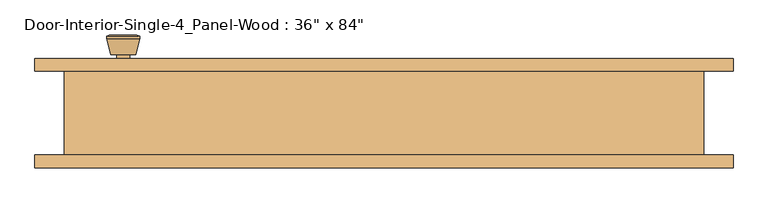
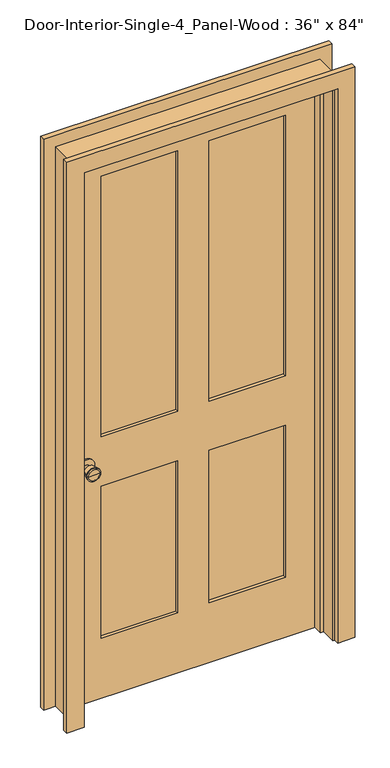
"""IFC4 building model written with IfcOpenShell, lengths in millimetres: door geometry."""

from ifc_helpers import new_model, si_unit, point, frame, frame_2d, origin, place, context, project, spatial, polyline, circle_curve, trimmed, segment, composite_curve, outline, extrude, faceted_brep, source, transform, mapped, element, save
from ifc_brep_helpers import plane_surface, cylinder_surface, revolved_surface, advanced_brep


def door_68a706ac(model_context):
    return source(origin(), model_context, "Body", "SolidModel", [
        advanced_brep(
        [(-393.7, 19.4, 914.4), (-383.7, 19.4, 914.4), (-403.7, 19.4, 914.4), (-373.2241324, -29.6, 914.4), (-393.7, -29.6, 914.4), (-414.1758676, -29.6, 914.4), (-368.7, -27.7721319, 914.4), (-418.7, -27.7721319, 914.4), (-368.7, -24.3084537, 914.4), (-418.7, -24.3084537, 914.4), (-375.063764, 0.4, 914.4), (-412.336236, 0.4, 914.4), (-383.7, 0.4, 914.4), (-403.7, 0.4, 914.4)],
        [
            (0, 1),
            (1, 2, circle_curve(frame((-393.7, 19.4, 914.4), z_axis=(0.0, 1.0, 0.0), x_axis=(-1.0, 0.0, 0.0)), 10.0)),
            (2, 0),
            (2, 1, circle_curve(frame((-393.7, 19.4, 914.4), z_axis=(0.0, 1.0, 0.0), x_axis=(-1.0, 0.0, 0.0)), 10.0)),
            (3, 4),
            (4, 5),
            (5, 3, circle_curve(frame((-393.7, -29.6, 914.4), z_axis=(0.0, -1.0, 0.0), x_axis=(-1.0, 0.0, 0.0)), 20.4758676)),
            (3, 5, circle_curve(frame((-393.7, -29.6, 914.4), z_axis=(0.0, -1.0, 0.0), x_axis=(-1.0, 0.0, 0.0)), 20.4758676)),
            (6, 3),
            (5, 7),
            (7, 6, circle_curve(frame((-393.7, -27.7721319, 914.4), z_axis=(0.0, -1.0, 0.0), x_axis=(-1.0, 0.0, 0.0)), 25.0)),
            (6, 7, circle_curve(frame((-393.7, -27.7721319, 914.4), z_axis=(0.0, -1.0, 0.0), x_axis=(-1.0, 0.0, 0.0)), 25.0)),
            (8, 6),
            (7, 9),
            (9, 8, circle_curve(frame((-393.7, -24.3084537, 914.4), z_axis=(0.0, -1.0, 0.0), x_axis=(-1.0, 0.0, 0.0)), 25.0)),
            (8, 9, circle_curve(frame((-393.7, -24.3084537, 914.4), z_axis=(0.0, -1.0, 0.0), x_axis=(-1.0, 0.0, 0.0)), 25.0)),
            (10, 8),
            (9, 11),
            (11, 10, circle_curve(frame((-393.7, 0.4, 914.4), z_axis=(0.0, -1.0, 0.0), x_axis=(-1.0, 0.0, 0.0)), 18.636236)),
            (10, 11, circle_curve(frame((-393.7, 0.4, 914.4), z_axis=(0.0, -1.0, 0.0), x_axis=(-1.0, 0.0, 0.0)), 18.636236)),
            (12, 10),
            (11, 13),
            (13, 12, circle_curve(frame((-393.7, 0.4, 914.4), z_axis=(0.0, -1.0, 0.0), x_axis=(-1.0, 0.0, 0.0)), 10.0)),
            (12, 13, circle_curve(frame((-393.7, 0.4, 914.4), z_axis=(0.0, -1.0, 0.0), x_axis=(-1.0, 0.0, 0.0)), 10.0)),
            (1, 12),
            (13, 2),
        ],
        [
            plane_surface(frame((-393.7, 19.4, 914.4), z_axis=(0.0, 1.0, 0.0), x_axis=(-1.0, 0.0, 0.0))),
            plane_surface(frame((-393.7, -29.6, 914.4), z_axis=(0.0, -1.0, 0.0), x_axis=(-1.0, 0.0, 0.0))),
            revolved_surface(polyline([(-414.1758676, -29.6, 914.4), (-418.7, -27.7721319, 914.4)]), (-393.7, 19.4, 914.4), (0.0, 1.0, 0.0)),
            cylinder_surface(frame((-393.7, 19.4, 914.4), z_axis=(0.0, 1.0, 0.0), x_axis=(-1.0, 0.0, 0.0)), 25.0),
            revolved_surface(polyline([(-418.7, -24.3084537, 914.4), (-412.336236, 0.4, 914.4)]), (-393.7, 19.4, 914.4), (0.0, 1.0, 0.0)),
            plane_surface(frame((-393.7, 0.4, 914.4), z_axis=(0.0, 1.0, 0.0), x_axis=(-1.0, 0.0, 0.0))),
            cylinder_surface(frame((-393.7, 19.4, 914.4), z_axis=(0.0, 1.0, 0.0), x_axis=(-1.0, 0.0, 0.0)), 10.0),
        ],
        [
            (0, [[1, 2, 3]]),
            (0, [[-3, 4, -1]]),
            (1, [[5, 6, 7]]),
            (1, [[-6, -5, 8]]),
            (2, [[9, -7, 10, 11]]),
            (2, [[-10, -8, -9, 12]]),
            (3, [[13, -11, 14, 15]]),
            (3, [[-14, -12, -13, 16]]),
            (4, [[17, -15, 18, 19]]),
            (4, [[-18, -16, -17, 20]]),
            (5, [[21, -19, 22, 23]]),
            (5, [[-22, -20, -21, 24]]),
            (6, [[25, -23, 26, -2]]),
            (6, [[-26, -24, -25, -4]]),
        ],
    ),
        extrude(outline(composite_curve([segment(trimmed(circle_curve(frame_2d((914.4, -393.7)), 30.0), [point((914.4, -423.7))], [point((914.4, -363.7))], False, "CARTESIAN"), True, "CONTINUOUS"), segment(trimmed(circle_curve(frame_2d((914.4, -393.7)), 30.0), [point((914.4, -363.7))], [point((914.4, -423.7))], False, "CARTESIAN"), True, "CONTINUOUS")], self_intersect=False)), frame((0.0, 19.4, 0.0), z_axis=(0.0, 1.0, 0.0), x_axis=(0.0, 0.0, 1.0)), (0.0, 0.0, 1.0), 6.0),
        advanced_brep(
        [(-393.7, 66.325, 914.4), (-403.7, 66.325, 914.4), (-383.7, 66.325, 914.4), (-373.2241324, 115.325, 914.4), (-414.1758676, 115.325, 914.4), (-393.7, 115.325, 914.4), (-368.7, 113.4971319, 914.4), (-418.7, 113.4971319, 914.4), (-368.7, 110.0334537, 914.4), (-418.7, 110.0334537, 914.4), (-375.063764, 85.325, 914.4), (-412.336236, 85.325, 914.4), (-383.7, 85.325, 914.4), (-403.7, 85.325, 914.4)],
        [
            (0, 1),
            (1, 2, circle_curve(frame((-393.7, 66.325, 914.4), z_axis=(0.0, -1.0, 0.0), x_axis=(-1.0, 0.0, 0.0)), 10.0)),
            (2, 0),
            (2, 1, circle_curve(frame((-393.7, 66.325, 914.4), z_axis=(0.0, -1.0, 0.0), x_axis=(-1.0, 0.0, 0.0)), 10.0)),
            (3, 4, circle_curve(frame((-393.7, 115.325, 914.4), z_axis=(0.0, 1.0, 0.0), x_axis=(-1.0, 0.0, 0.0)), 20.4758676)),
            (4, 5),
            (5, 3),
            (4, 3, circle_curve(frame((-393.7, 115.325, 914.4), z_axis=(0.0, 1.0, 0.0), x_axis=(-1.0, 0.0, 0.0)), 20.4758676)),
            (6, 7, circle_curve(frame((-393.7, 113.4971319, 914.4), z_axis=(0.0, 1.0, 0.0), x_axis=(-1.0, 0.0, 0.0)), 25.0)),
            (7, 4),
            (3, 6),
            (7, 6, circle_curve(frame((-393.7, 113.4971319, 914.4), z_axis=(0.0, 1.0, 0.0), x_axis=(-1.0, 0.0, 0.0)), 25.0)),
            (8, 9, circle_curve(frame((-393.7, 110.0334537, 914.4), z_axis=(0.0, 1.0, 0.0), x_axis=(-1.0, 0.0, 0.0)), 25.0)),
            (9, 7),
            (6, 8),
            (9, 8, circle_curve(frame((-393.7, 110.0334537, 914.4), z_axis=(0.0, 1.0, 0.0), x_axis=(-1.0, 0.0, 0.0)), 25.0)),
            (10, 11, circle_curve(frame((-393.7, 85.325, 914.4), z_axis=(0.0, 1.0, 0.0), x_axis=(-1.0, 0.0, 0.0)), 18.636236)),
            (11, 9),
            (8, 10),
            (11, 10, circle_curve(frame((-393.7, 85.325, 914.4), z_axis=(0.0, 1.0, 0.0), x_axis=(-1.0, 0.0, 0.0)), 18.636236)),
            (12, 13, circle_curve(frame((-393.7, 85.325, 914.4), z_axis=(0.0, 1.0, 0.0), x_axis=(-1.0, 0.0, 0.0)), 10.0)),
            (13, 11),
            (10, 12),
            (13, 12, circle_curve(frame((-393.7, 85.325, 914.4), z_axis=(0.0, 1.0, 0.0), x_axis=(-1.0, 0.0, 0.0)), 10.0)),
            (1, 13),
            (12, 2),
        ],
        [
            plane_surface(frame((-393.7, 66.325, 914.4), z_axis=(0.0, -1.0, 0.0), x_axis=(-1.0, 0.0, 0.0))),
            plane_surface(frame((-393.7, 115.325, 914.4), z_axis=(0.0, 1.0, 0.0), x_axis=(-1.0, 0.0, 0.0))),
            revolved_surface(polyline([(-414.1758676, 115.325, 914.4), (-418.7, 113.4971319, 914.4)]), (-393.7, 66.325, 914.4), (0.0, -1.0, 0.0)),
            cylinder_surface(frame((-393.7, 66.325, 914.4), z_axis=(0.0, -1.0, 0.0), x_axis=(-1.0, 0.0, 0.0)), 25.0),
            revolved_surface(polyline([(-418.7, 110.0334537, 914.4), (-412.336236, 85.325, 914.4)]), (-393.7, 66.325, 914.4), (0.0, -1.0, 0.0)),
            plane_surface(frame((-393.7, 85.325, 914.4), z_axis=(0.0, -1.0, 0.0), x_axis=(-1.0, 0.0, 0.0))),
            cylinder_surface(frame((-393.7, 66.325, 914.4), z_axis=(0.0, -1.0, 0.0), x_axis=(-1.0, 0.0, 0.0)), 10.0),
        ],
        [
            (0, [[1, 2, 3]]),
            (0, [[-3, 4, -1]]),
            (1, [[5, 6, 7]]),
            (1, [[8, -7, -6]]),
            (2, [[9, 10, -5, 11]]),
            (2, [[12, -11, -8, -10]]),
            (3, [[13, 14, -9, 15]]),
            (3, [[16, -15, -12, -14]]),
            (4, [[17, 18, -13, 19]]),
            (4, [[20, -19, -16, -18]]),
            (5, [[21, 22, -17, 23]]),
            (5, [[24, -23, -20, -22]]),
            (6, [[-2, 25, -21, 26]]),
            (6, [[-4, -26, -24, -25]]),
        ],
    ),
        extrude(outline(composite_curve([segment(trimmed(circle_curve(frame_2d((914.4, -393.7)), 30.0), [point((914.4, -423.7))], [point((914.4, -363.7))], False, "CARTESIAN"), True, "CONTINUOUS"), segment(trimmed(circle_curve(frame_2d((914.4, -393.7)), 30.0), [point((914.4, -363.7))], [point((914.4, -423.7))], False, "CARTESIAN"), True, "CONTINUOUS")], self_intersect=False)), frame((0.0, 60.325, 0.0), z_axis=(0.0, 1.0, 0.0), x_axis=(0.0, 0.0, 1.0)), (0.0, 0.0, 1.0), 6.0),
        faceted_brep([(482.6, 60.325, 0.0), (482.6, -66.675, 0.0), (457.2, -66.675, 0.0), (457.2, -9.525, 0.0), (444.5, -9.525, 0.0), (444.5, 25.4, 0.0), (457.2, 25.4, 0.0), (457.2, 60.325, 0.0), (482.6, 60.325, 2159.0), (482.6, -66.675, 2159.0), (-482.6, -66.675, 2159.0), (-482.6, -66.675, 0.0), (-457.2, -66.675, 0.0), (-457.2, -66.675, 2133.6), (457.2, -66.675, 2133.6), (457.2, -9.525, 2133.6), (-457.2, -9.525, 2133.6), (-457.2, -9.525, 0.0), (-444.5, -9.525, 0.0), (-444.5, -9.525, 2120.9), (444.5, -9.525, 2120.9), (444.5, 25.4, 2120.9), (-444.5, 25.4, 2120.9), (-444.5, 25.4, 0.0), (-457.2, 25.4, 0.0), (-457.2, 25.4, 2133.6), (457.2, 25.4, 2133.6), (457.2, 60.325, 2133.6), (-457.2, 60.325, 2133.6), (-457.2, 60.325, 0.0), (-482.6, 60.325, 0.0), (-482.6, 60.325, 2159.0)], [[[0, 1, 2, 3, 4, 5, 6, 7]], [[1, 0, 8, 9]], [[2, 1, 9, 10, 11, 12, 13, 14]], [[3, 2, 14, 15]], [[4, 3, 15, 16, 17, 18, 19, 20]], [[5, 4, 20, 21]], [[6, 5, 21, 22, 23, 24, 25, 26]], [[7, 6, 26, 27]], [[0, 7, 27, 28, 29, 30, 31, 8]], [[9, 8, 31, 10]], [[15, 14, 13, 16]], [[21, 20, 19, 22]], [[27, 26, 25, 28]], [[30, 29, 24, 23, 18, 17, 12, 11]], [[10, 31, 30, 11]], [[16, 13, 12, 17]], [[22, 19, 18, 23]], [[28, 25, 24, 29]]]),
        extrude(outline(polyline([(2133.6, -457.2), (0.0, -457.2), (0.0, 457.2), (2133.6, 457.2), (2133.6, -457.2)]), holes=[polyline([(2014.5375, 57.15), (2014.5375, 336.55), (1009.65, 336.55), (1009.65, 57.15), (2014.5375, 57.15)]), polyline([(1009.65, -57.15), (1009.65, -336.55), (2014.5375, -336.55), (2014.5375, -57.15), (1009.65, -57.15)]), polyline([(819.15, 57.15), (819.15, 336.55), (231.775, 336.55), (231.775, 57.15), (819.15, 57.15)]), polyline([(231.775, -57.15), (231.775, -336.55), (819.15, -336.55), (819.15, -57.15), (231.775, -57.15)])]), frame((0.0, 25.4, 0.0), z_axis=(0.0, 1.0, 0.0), x_axis=(0.0, 0.0, 1.0)), (0.0, 0.0, 1.0), 34.925),
        extrude(outline(polyline([(336.55, 37.0416667), (57.15, 37.0416667), (57.15, 48.6833333), (336.55, 48.6833333), (336.55, 37.0416667)])), frame((0.0, 0.0, 1009.65), z_axis=(0.0, 0.0, 1.0), x_axis=(1.0, 0.0, 0.0)), (0.0, 0.0, 1.0), 1004.8875),
        extrude(outline(polyline([(-57.15, 37.0416667), (-336.55, 37.0416667), (-336.55, 48.6833333), (-57.15, 48.6833333), (-57.15, 37.0416667)])), frame((0.0, 0.0, 1009.65), z_axis=(0.0, 0.0, 1.0), x_axis=(1.0, 0.0, 0.0)), (0.0, 0.0, 1.0), 1004.8875),
        extrude(outline(polyline([(336.55, 37.0416667), (57.15, 37.0416667), (57.15, 48.6833333), (336.55, 48.6833333), (336.55, 37.0416667)])), frame((0.0, 0.0, 231.775), z_axis=(0.0, 0.0, 1.0), x_axis=(1.0, 0.0, 0.0)), (0.0, 0.0, 1.0), 587.375),
        extrude(outline(polyline([(-57.15, 37.0416667), (-336.55, 37.0416667), (-336.55, 48.6833333), (-57.15, 48.6833333), (-57.15, 37.0416667)])), frame((0.0, 0.0, 231.775), z_axis=(0.0, 0.0, 1.0), x_axis=(1.0, 0.0, 0.0)), (0.0, 0.0, 1.0), 587.375),
        extrude(outline(polyline([(0.0, 463.55), (0.0, 527.05), (2203.45, 527.05), (2203.45, -527.05), (0.0, -527.05), (0.0, -463.55), (2139.95, -463.55), (2139.95, 463.55), (0.0, 463.55)])), frame((0.0, 60.325, 0.0), z_axis=(0.0, 1.0, 0.0), x_axis=(0.0, 0.0, 1.0)), (0.0, 0.0, 1.0), 19.05),
        extrude(outline(polyline([(0.0, 463.55), (0.0, 527.05), (2203.45, 527.05), (2203.45, -527.05), (0.0, -527.05), (0.0, -463.55), (2139.95, -463.55), (2139.95, 463.55), (0.0, 463.55)])), frame((0.0, -85.725, 0.0), z_axis=(0.0, 1.0, 0.0), x_axis=(0.0, 0.0, 1.0)), (0.0, 0.0, 1.0), 19.05),
    ])


if __name__ == "__main__":
    model = new_model("IFC4")
    model_context = context("Model", 3, world=origin())
    ifc_project = project(units=[si_unit("LENGTHUNIT", "METRE", prefix="MILLI")], contexts=[model_context])
    site = spatial("IfcSite", under=ifc_project)
    building = spatial("IfcBuilding", under=site)
    placement = place(None, origin())
    door_shape = door_68a706ac(model_context)
    element("IfcDoor", 1, ObjectType="Door-Interior-Single-4_Panel-Wood : 36\" x 84\"", at=placement, inside=building, context=model_context, shape_type="MappedRepresentation", body=[
        mapped(door_shape, transform((0.0, 0.0, 0.0), x_axis=(1.0, 0.0, 0.0), y_axis=(0.0, 1.0, 0.0), z_axis=(0.0, 0.0, 1.0))),
    ])
    save(model, "model.ifc")

# Revit data of these elements
# Type "Door-Interior-Single-4_Panel-Wood : 36\" x 84\""
#   Type Mark = "9"
#   Assembly Code = "C1020300"
#   Analytic Construction = "Wooden"
#   Top Rail = 0' - 4 11/16"
#   Thickness = 0' - 1 3/8"
#   Thermal Resistance (R) = 2.5876 (h·ft²·°F)/BTU
#   Swing Angle [instance default] = 90.00°
#   Stiles = 0' - 4 3/4"
#   Rough Width = 3' - 2"
#   Rough Height = 7' - 1"
#   Mullion = 0' - 4 1/2"
#   Lock Rail = 0' - 7 1/2"
#   Height = 7' - 0"
#   Width = 3' - 0"
#   Heat Transfer Coefficient (U) = 0.3865 BTU/(h·ft²·°F)
#   Bottom Rail = 0' - 9 1/8"
#   Trim Material = Cherry
#   Panel Material = Cherry
#   Frame Material = Cherry
#   Door Handle Material = Aluminum
#   Visual Light Transmittance = 0
#   Solar Heat Gain Coefficient = 0
#   Wall Closure = (empty or 0)
#   Function = (empty or 0)
# Element 1 (IfcDoor, "Door-Interior-Single-4_Panel-Wood : 36\" x 84\"")
#   Materials on its faces: "Cherry", "Aluminum"
# Materials
#   "Cherry": class "Wood", colour RGB 226 177 128, transparency 0, Description = "Prunus Serotina", Cost = 0
#   "Aluminum": class "Metal", colour RGB 247 247 247, transparency 0, Description = "Aluminum 6061", Cost = 0
